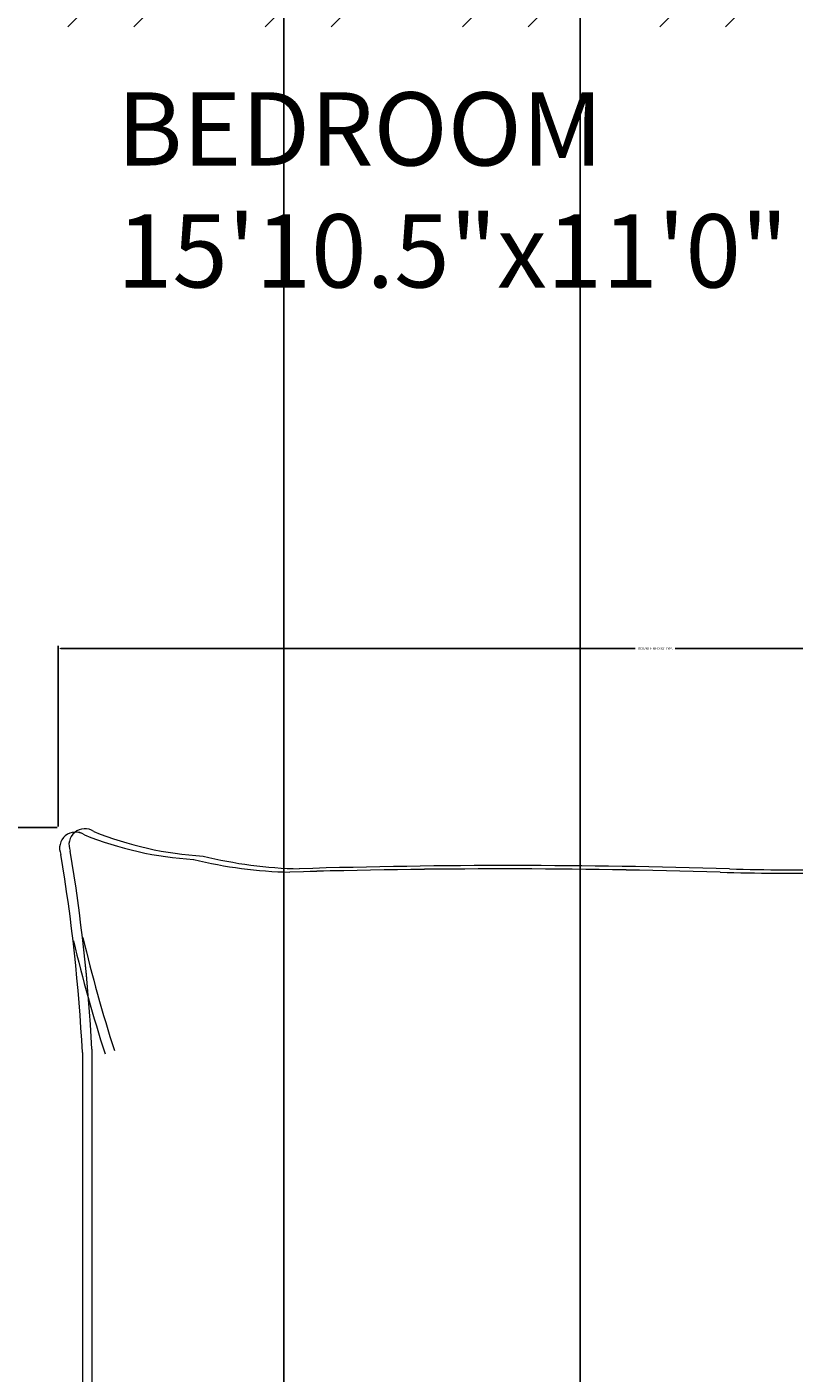
# Model space of a CAD drawing. Units: inches. Extents: x 1601 to 2297, y 1496 to 2631.
# Tile 21 of 57: x 2140 to 2193, y 1701 to 1793. Entities that reach past the tile are written whole.
import ezdxf

# ---------------------------------------------------------------- set-up
doc = ezdxf.new("R2010")
doc.units = ezdxf.units.IN
for name, color, linetype, lineweight in [('A-ANNO-DIMS', 2, 'Continuous', 18), ('A-AREA-IDEN', 7, 'Continuous', 18), ('A-FURN', 8, 'Continuous', 18), ('A-WALL-PATT', 215, 'Continuous', 13)]:
    doc.layers.add(name, color=color, linetype=linetype, lineweight=lineweight)
doc.styles.get("Standard").update_dxf_attribs({"font": 'arial.ttf'})
doc.dimstyles.get("Standard").update_dxf_attribs({"dimtxt": 0.18, "dimasz": 0.18, "dimexe": 0.18, "dimexo": 0.0625, "dimgap": 0.09, "dimtad": 0, "dimtih": 1, "dimtoh": 1, "dimdec": 4, "dimzin": 0, "dimdsep": 46, "dimtxsty": 'Standard', "dimcen": 0.09, "dimadec": 0, "dimazin": 0, "dimtfac": 1, "dimtdec": 4, "dimtofl": 0, "dimtmove": 0, "dimatfit": 3, "dimfxl": 1, "dimtolj": 1, "dimtzin": 0, "dimarcsym": 0})

# ---------------------------------------------------------------- blocks, each defined once
blk = doc.blocks.new('BED-DOUBLE')
for p, q in [((79.245, 15.063), (79.245, 39.677)), ((79.245, 15.063), (79.245, 39.677)), ((79.245, 15.063), (79.245, 39.677)), ((79.245, 15.063), (79.245, 39.677)), ((79.884, 15.292), (79.884, 39.905)), ((79.884, 15.291), (79.884, 39.905)), ((79.884, 15.292), (79.884, 39.905)), ((79.884, 15.291), (79.884, 39.905))]:
    blk.add_line(p, q)
for centre, radius, start, end in [((-23.712, -17.222), 106.459, 13.38322, 17.70533), ((-23.712, -17.222), 106.459, 13.38322, 17.70533), ((-23.712, -17.222), 106.459, 13.38322, 17.70533), ((-23.712, -17.222), 106.459, 13.38322, 17.70533), ((-23.073, -16.994), 106.459, 13.38322, 17.70533), ((-23.073, -16.994), 106.459, 13.38322, 17.70533), ((-23.073, -16.994), 106.459, 13.38322, 17.70533), ((-23.073, -16.994), 106.459, 13.38322, 17.70533), ((200.837, 21.427), 121.759, 182.99578, 189.40907), ((200.837, 21.426), 121.759, 182.99578, 189.40907), ((200.837, 21.427), 121.759, 182.99578, 189.40907), ((200.837, 21.426), 121.759, 182.99578, 189.40907), ((201.476, 21.655), 121.759, 182.99578, 189.40907), ((201.476, 21.655), 121.759, 182.99578, 189.40907), ((201.476, 21.655), 121.759, 182.99578, 189.40907), ((201.476, 21.655), 121.759, 182.99578, 189.40907), ((31.174, -167.308), 170.11, 88.4762, 91.00819), ((31.174, -167.308), 170.11, 88.4762, 91.00819), ((31.174, -167.308), 170.11, 88.4762, 91.00819), ((31.174, -167.308), 170.11, 88.4762, 91.00819), ((31.813, -167.079), 170.11, 88.4762, 91.00819), ((31.813, -167.08), 170.11, 88.4762, 91.00819), ((31.813, -167.079), 170.11, 88.4762, 91.00819), ((31.813, -167.08), 170.11, 88.4762, 91.00819), ((51.253, 485.051), 482.31, 268.22771, 271.71854), ((51.253, 485.05), 482.31, 268.22771, 271.71854), ((51.253, 485.051), 482.31, 268.22771, 271.71854), ((51.253, 485.05), 482.31, 268.22771, 271.71854), ((65.154, -26.671), 29.634, 76.06484, 88.91125), ((65.154, -26.672), 29.634, 76.06484, 88.91125), ((65.154, -26.671), 29.634, 76.06484, 88.91125), ((65.154, -26.672), 29.634, 76.06484, 88.91125), ((50.614, 484.822), 482.31, 268.22771, 271.71854), ((50.614, 484.822), 482.31, 268.22771, 271.71854), ((50.614, 484.822), 482.31, 268.22771, 271.71854), ((50.614, 484.822), 482.31, 268.22771, 271.71854), ((64.515, -26.9), 29.634, 76.06484, 88.91125), ((64.515, -26.9), 29.634, 76.06484, 88.91125), ((64.515, -26.9), 29.634, 76.06484, 88.91125), ((64.515, -26.9), 29.634, 76.06484, 88.91125), ((70.276, -21.66), 23.562, 67.97508, 86.652), ((70.276, -21.66), 23.562, 67.97508, 86.652), ((70.276, -21.66), 23.562, 67.97508, 86.652), ((70.276, -21.66), 23.562, 67.97508, 86.652), ((70.915, -21.431), 23.562, 67.97508, 86.652), ((70.915, -21.432), 23.562, 67.97508, 86.652), ((70.915, -21.431), 23.562, 67.97508, 86.652), ((70.915, -21.432), 23.562, 67.97508, 86.652), ((79.718, 1.087), 1.089, 236.17358, 23.47814), ((79.718, 1.087), 1.089, 236.17358, 23.47814), ((79.718, 1.087), 1.089, 236.17358, 23.47814), ((79.718, 1.087), 1.089, 236.17358, 23.47814), ((80.357, 1.316), 1.089, 236.17358, 23.47814), ((80.357, 1.316), 1.089, 236.17358, 23.47814), ((80.357, 1.315), 1.089, 236.17358, 23.47814), ((80.357, 1.315), 1.089, 236.17358, 23.47814)]:
    blk.add_arc(centre, radius, start, end)
blk = doc.blocks.new('*D12')
at = {"layer": 'A-ANNO-DIMS', "color": 0, "lineweight": -2, "transparency": 16777216}
for p, q in [((2142.379, 1738.191), (2142.379, 1750.54)), ((2142.559, 1750.36), (2181.784, 1750.36)), ((2223.747, 1750.36), (2184.522, 1750.36)), ((2223.927, 1738.191), (2223.927, 1750.54))]:
    blk.add_line(p, q, dxfattribs=at)
at = {"layer": 'A-ANNO-DIMS', "color": 0, "transparency": 16777216}
for points in [[(2142.559, 1750.39), (2142.559, 1750.33), (2142.379, 1750.36)], [(2223.747, 1750.39), (2223.747, 1750.33), (2223.927, 1750.36)]]:
    blk.add_solid(points, dxfattribs=at)
at = {"layer": 'Defpoints', "color": 0, "transparency": 16777216}
for p in [(2142.379, 1750.36), (2142.379, 1738.128), (2223.927, 1738.128)]:
    blk.add_point(p, dxfattribs=at)
at = {"layer": 'A-ANNO-DIMS', "color": 0, "transparency": 16777216, "insert": (2183.153, 1750.36), "char_height": 0.18, "attachment_point": 5}
blk.add_mtext('\\A1;DOUBLE BED 82 TYP.', dxfattribs=at)
blk = doc.blocks.new('*D13')
at = {"layer": 'A-ANNO-DIMS', "color": 0, "lineweight": -2, "transparency": 16777216}
for p, q in [((2142.316, 1738.128), (2129.966, 1738.128)), ((2130.146, 1737.948), (2130.146, 1710.398)), ((2130.146, 1682.484), (2130.146, 1710.034)), ((2142.316, 1682.304), (2129.966, 1682.304))]:
    blk.add_line(p, q, dxfattribs=at)
at = {"layer": 'A-ANNO-DIMS', "color": 0, "transparency": 16777216}
for points in [[(2130.116, 1737.948), (2130.176, 1737.948), (2130.146, 1738.128)], [(2130.116, 1682.484), (2130.176, 1682.484), (2130.146, 1682.304)]]:
    blk.add_solid(points, dxfattribs=at)
at = {"layer": 'Defpoints', "color": 0, "transparency": 16777216}
for p in [(2142.379, 1738.128), (2130.146, 1682.304), (2142.379, 1682.304)]:
    blk.add_point(p, dxfattribs=at)
at = {"layer": 'A-ANNO-DIMS', "color": 0, "transparency": 16777216, "insert": (2130.146, 1710.216), "char_height": 0.18, "attachment_point": 5}
blk.add_mtext('\\A1;56 TYP.', dxfattribs=at)
blk = doc.blocks.new('*D38')
at = {"layer": 'A-ANNO-DIMS', "color": 0, "lineweight": -2, "transparency": 16777216}
for p, q in [((2178.037, 2085.263), (2178.037, 1513.748)), ((2157.799, 2066.513), (2157.799, 1513.748)), ((2157.979, 1513.928), (2167.523, 1513.928)), ((2177.857, 1513.928), (2168.313, 1513.928))]:
    blk.add_line(p, q, dxfattribs=at)
at = {"layer": 'A-ANNO-DIMS', "color": 0, "transparency": 16777216}
for points in [[(2157.979, 1513.958), (2157.979, 1513.898), (2157.799, 1513.928)], [(2177.857, 1513.958), (2177.857, 1513.898), (2178.037, 1513.928)]]:
    blk.add_solid(points, dxfattribs=at)
at = {"layer": 'Defpoints', "color": 0, "transparency": 16777216}
for p in [(2178.037, 2085.325), (2157.799, 2066.575), (2178.037, 1513.928)]:
    blk.add_point(p, dxfattribs=at)
at = {"layer": 'A-ANNO-DIMS', "color": 0, "transparency": 16777216, "insert": (2167.918, 1513.928), "char_height": 0.18, "attachment_point": 5}
blk.add_mtext('\\A1;20.24', dxfattribs=at)

msp = doc.modelspace()

# ---------------------------------------------------------------- hatches: boundary and pattern name
at = {"layer": 'A-WALL-PATT'}
h = msp.add_hatch(dxfattribs=at)
h.set_pattern_fill('ANSI32', color=256)
h.paths.add_polyline_path([(1842.0336, 2528.0767), (1842.0336, 2532.3254), (1686.0373, 2532.3254), (1686.0373, 2492.9493), (1695.0373, 2492.9493), (1695.0373, 2523.3254), (1827.0373, 2523.3254), (1827.0373, 2416.8254), (1834.6225, 2416.8254), (1834.6225, 2419.0754), (1834.6225, 2421.3254), (1831.5373, 2421.3254), (1831.5373, 2523.3254), (1842.0336, 2523.3254)])
h.paths.add_polyline_path([(1695.0373, 2432.9493), (1686.0373, 2432.9493), (1686.0373, 2325.989), (1695.0373, 2325.989), (1695.0373, 2347.8254), (1827.0373, 2347.8254), (1827.0373, 2287.8254), (1823.2991, 2287.8254), (1823.2991, 2283.3254), (1847.9422, 2283.3254), (1847.9422, 2285.5754), (1847.9422, 2287.8254), (1831.5373, 2287.8254), (1831.5373, 2347.8254), (1846.9946, 2347.8254), (1846.9946, 2350.0754), (1846.9946, 2352.3254), (1695.0373, 2352.3254)])
h.paths.add_polyline_path([(1807.1169, 1573.5395), (2055.0405, 1573.5395), (2055.0405, 1610.6322), (1807.1169, 1610.6322)], flags=9)
h.paths.add_polyline_path([(1841.1631, 1712.7967), (1870.3957, 1712.7967), (1870.3957, 1731.454), (1841.1631, 1731.454)], flags=9)
h.paths.add_polyline_path([(2144.3862, 1772.185), (2191.0233, 1772.185), (2191.0233, 1790.8423), (2144.3862, 1790.8423)], flags=9)
h.paths.add_polyline_path([(2143.0128, 1827.3312), (2177.9958, 1827.3312), (2177.9958, 1845.9886), (2143.0128, 1845.9886)], flags=9)
h.paths.add_polyline_path([(2041.2439, 1833.5691), (2070.8516, 1833.5691), (2070.8516, 1852.2264), (2041.2439, 1852.2264)], flags=9)
h.paths.add_polyline_path([(2097.2791, 1947.0598), (2134.2061, 1947.0598), (2134.2061, 1965.7171), (2097.2791, 1965.7171)], flags=9)
h.paths.add_polyline_path([(2214.995, 1904.3124), (2214.995, 1942.2899), (2196.3376, 1942.2899), (2196.3376, 1904.3124)], flags=9)
h.paths.add_polyline_path([(2186.6284, 2043.8031), (2219.7935, 2043.8031), (2219.7935, 2062.4605), (2186.6284, 2062.4605)], flags=9)
h.paths.add_polyline_path([(2064.0877, 2031.616), (2097.4949, 2031.616), (2097.4949, 2050.2734), (2064.0877, 2050.2734)], flags=9)
h.paths.add_polyline_path([(1973.1349, 1986.0688), (2008.4009, 1986.0688), (2008.4009, 2004.7261), (1973.1349, 2004.7261)], flags=9)
h.paths.add_polyline_path([(1976.3676, 2106.9635), (2005.7469, 2106.9635), (2005.7469, 2125.6209), (1976.3676, 2125.6209)], flags=9)
h.paths.add_polyline_path([(1991.7852, 2180.4863), (2027.0513, 2180.4863), (2027.0513, 2199.1437), (1991.7852, 2199.1437)], flags=9)
h.paths.add_polyline_path([(2106.1801, 2187.9359), (2152.2101, 2187.9359), (2152.2101, 2206.5932), (2106.1801, 2206.5932)], flags=9)
h.paths.add_polyline_path([(2148.6686, 2262.2542), (2182.318, 2262.2542), (2182.318, 2280.9115), (2148.6686, 2280.9115)], flags=9)
h.paths.add_polyline_path([(2041.6327, 2252.8147), (2071.2405, 2252.8147), (2071.2405, 2271.4721), (2041.6327, 2271.4721)], flags=9)
h.paths.add_polyline_path([(2063.9734, 2375.4265), (2100.9004, 2375.4265), (2100.9004, 2394.0839), (2063.9734, 2394.0839)], flags=9)
h.paths.add_polyline_path([(2216.4955, 2330.9748), (2216.4955, 2370.2654), (2197.8381, 2370.2654), (2197.8381, 2330.9748)], flags=9)
h.paths.add_polyline_path([(2179.1416, 2485.8687), (2212.3067, 2485.8687), (2212.3067, 2504.5261), (2179.1416, 2504.5261)], flags=9)
h.paths.add_polyline_path([(2078.7442, 2471.1516), (2112.1514, 2471.1516), (2112.1514, 2489.809), (2078.7442, 2489.809)], flags=9)
h.paths.add_polyline_path([(1915.9631, 2329.4668), (1952.8902, 2329.4668), (1952.8902, 2348.1241), (1915.9631, 2348.1241)], flags=9)
h.paths.add_polyline_path([(1904.3189, 2499.6709), (1940.4512, 2499.6709), (1940.4512, 2518.3282), (1904.3189, 2518.3282)], flags=9)
h.paths.add_polyline_path([(1892.3665, 2100.4595), (1925.6374, 2100.4595), (1925.6374, 2119.1169), (1892.3665, 2119.1169)], flags=9)
h.paths.add_polyline_path([(1909.2984, 1805.9631), (1946.2254, 1805.9631), (1946.2254, 1824.6205), (1909.2984, 1824.6205)], flags=9)
h.paths.add_polyline_path([(1934.6056, 1658.616), (1970.738, 1658.616), (1970.738, 1677.2733), (1934.6056, 1677.2733)], flags=9)
h.paths.add_polyline_path([(1711.2052, 1789.8902), (1750.0456, 1789.8902), (1750.0456, 1808.5476), (1711.2052, 1808.5476)], flags=9)
h.paths.add_polyline_path([(1742.7874, 1854.6743), (1771.9449, 1854.6743), (1771.9449, 1873.3317), (1742.7874, 1873.3317)], flags=9)
h.paths.add_polyline_path([(1807.3592, 1997.7912), (1850.1116, 1997.7912), (1850.1116, 2016.4486), (1807.3592, 2016.4486)], flags=9)
h.paths.add_polyline_path([(1717.4579, 2237.7844), (1760.2103, 2237.7844), (1760.2103, 2256.4417), (1717.4579, 2256.4417)], flags=9)
h.paths.add_polyline_path([(1780.9285, 2324.0623), (1810.086, 2324.0623), (1810.086, 2342.7197), (1780.9285, 2342.7197)], flags=25)
h.paths.add_polyline_path([(1837.696, 2449.2024), (1866.9286, 2449.2024), (1866.9286, 2467.8598), (1837.696, 2467.8598)], flags=9)
h.paths.add_polyline_path([(1712.7752, 2484.9404), (1751.6156, 2484.9404), (1751.6156, 2503.5977), (1712.7752, 2503.5977)], flags=25)
h = msp.add_hatch(dxfattribs=at)
h.set_pattern_fill('ANSI32', color=256)
h.paths.add_polyline_path([(1973.9371, 2211.3254), (1893.0373, 2211.3254), (1893.0373, 2287.8254), (1884.6167, 2287.8254), (1884.6167, 2285.5754), (1884.6167, 2283.3254), (1888.5373, 2283.3254), (1888.5373, 2145.3254), (1695.0373, 2145.3254), (1695.0373, 2173.8724), (1690.5373, 2173.8724), (1686.0373, 2173.8724), (1686.0373, 2136.3254), (1722.5687, 2136.3254), (1722.5687, 2117.4352), (1731.5687, 2117.4352), (1731.5687, 2136.3254), (1893.0373, 2136.3254), (1893.0373, 2202.3254), (1959.0373, 2202.3254), (1959.0373, 2182.1303), (1968.0373, 2182.1303), (1968.0373, 2202.3254), (1973.9371, 2202.3254)])
h.paths.add_polyline_path([(2094.0373, 2274.6364), (2096.4294, 2274.6364), (2096.4294, 2276.8864), (2096.4294, 2279.1364), (2094.0373, 2279.1364), (2094.0373, 2290.8254), (2094.0373, 2295.3254), (2089.5373, 2295.3254), (2089.5373, 2230.8254), (2035.5373, 2230.8254), (2035.5373, 2299.8254), (2031.0373, 2299.8254), (2031.0373, 2211.3254), (2023.0065, 2211.3254), (2023.0065, 2202.3254), (2031.0373, 2202.3254), (2031.0373, 2140.8254), (1968.0373, 2140.8254), (1968.0373, 2145.9106), (1963.5373, 2145.9106), (1959.0373, 2145.9106), (1959.0373, 2116.839), (1963.5373, 2116.839), (1968.0373, 2116.839), (1968.0373, 2131.8254), (2031.0373, 2131.8254), (2031.0373, 2094.3254), (2031.0373, 2085.3254), (2031.0373, 2056.8254), (1968.0373, 2056.8254), (1968.0373, 2070.4947), (1963.5373, 2070.4947), (1959.0373, 2070.4947), (1959.0373, 2040.3029), (1968.0373, 2040.3029), (1968.0373, 2047.8254), (2031.0373, 2047.8254), (2031.0373, 1983.3254), (2031.0373, 1978.8254), (2021.1979, 1978.8254), (2021.1979, 1974.3254), (2031.0373, 1974.3254), (2031.0373, 1954.3528), (2035.5373, 1954.3528), (2035.5373, 1974.3254), (2035.5373, 1981.8254), (2055.5513, 1981.8254), (2055.5513, 1986.3254), (2035.5373, 1986.3254), (2035.5373, 2047.8254), (2040.0373, 2047.8254), (2040.0373, 2085.3254), (2040.0373, 2094.3254), (2040.0373, 2140.8254), (2035.5373, 2140.8254), (2035.5373, 2226.3254), (2089.5373, 2226.3254), (2094.0373, 2226.3254)])
h.paths.add_polyline_path([(2226.0373, 2230.8254), (2134.5373, 2230.8254), (2134.5373, 2233.5437), (2130.0373, 2233.5437), (2130.0373, 2226.3254), (2134.5373, 2226.3254), (2226.0373, 2226.3254)])
h.paths.add_polyline_path([(1807.1169, 1573.5395), (2055.0405, 1573.5395), (2055.0405, 1610.6322), (1807.1169, 1610.6322)], flags=9)
h.paths.add_polyline_path([(1841.1631, 1712.7967), (1870.3957, 1712.7967), (1870.3957, 1731.454), (1841.1631, 1731.454)], flags=9)
h.paths.add_polyline_path([(2144.3862, 1772.185), (2191.0233, 1772.185), (2191.0233, 1790.8423), (2144.3862, 1790.8423)], flags=9)
h.paths.add_polyline_path([(2143.0128, 1827.3312), (2177.9958, 1827.3312), (2177.9958, 1845.9886), (2143.0128, 1845.9886)], flags=9)
h.paths.add_polyline_path([(2041.2439, 1833.5691), (2070.8516, 1833.5691), (2070.8516, 1852.2264), (2041.2439, 1852.2264)], flags=9)
h.paths.add_polyline_path([(2097.2791, 1947.0598), (2134.2061, 1947.0598), (2134.2061, 1965.7171), (2097.2791, 1965.7171)], flags=9)
h.paths.add_polyline_path([(2214.995, 1904.3124), (2214.995, 1942.2899), (2196.3376, 1942.2899), (2196.3376, 1904.3124)], flags=9)
h.paths.add_polyline_path([(2186.6284, 2043.8031), (2219.7935, 2043.8031), (2219.7935, 2062.4605), (2186.6284, 2062.4605)], flags=9)
h.paths.add_polyline_path([(2064.0877, 2031.616), (2097.4949, 2031.616), (2097.4949, 2050.2734), (2064.0877, 2050.2734)], flags=9)
h.paths.add_polyline_path([(1973.1349, 1986.0688), (2008.4009, 1986.0688), (2008.4009, 2004.7261), (1973.1349, 2004.7261)], flags=25)
h.paths.add_polyline_path([(1976.3676, 2106.9635), (2005.7469, 2106.9635), (2005.7469, 2125.6209), (1976.3676, 2125.6209)], flags=25)
h.paths.add_polyline_path([(1991.7852, 2180.4863), (2027.0513, 2180.4863), (2027.0513, 2199.1437), (1991.7852, 2199.1437)], flags=25)
h.paths.add_polyline_path([(2106.1801, 2187.9359), (2152.2101, 2187.9359), (2152.2101, 2206.5932), (2106.1801, 2206.5932)], flags=9)
h.paths.add_polyline_path([(2148.6686, 2262.2542), (2182.318, 2262.2542), (2182.318, 2280.9115), (2148.6686, 2280.9115)], flags=9)
h.paths.add_polyline_path([(2041.6327, 2252.8147), (2071.2405, 2252.8147), (2071.2405, 2271.4721), (2041.6327, 2271.4721)], flags=25)
h.paths.add_polyline_path([(2063.9734, 2375.4265), (2100.9004, 2375.4265), (2100.9004, 2394.0839), (2063.9734, 2394.0839)], flags=9)
h.paths.add_polyline_path([(2216.4955, 2330.9748), (2216.4955, 2370.2654), (2197.8381, 2370.2654), (2197.8381, 2330.9748)], flags=9)
h.paths.add_polyline_path([(2179.1416, 2485.8687), (2212.3067, 2485.8687), (2212.3067, 2504.5261), (2179.1416, 2504.5261)], flags=9)
h.paths.add_polyline_path([(2078.7442, 2471.1516), (2112.1514, 2471.1516), (2112.1514, 2489.809), (2078.7442, 2489.809)], flags=9)
h.paths.add_polyline_path([(1915.9631, 2329.4668), (1952.8902, 2329.4668), (1952.8902, 2348.1241), (1915.9631, 2348.1241)], flags=9)
h.paths.add_polyline_path([(1904.3189, 2499.6709), (1940.4512, 2499.6709), (1940.4512, 2518.3282), (1904.3189, 2518.3282)], flags=9)
h.paths.add_polyline_path([(1892.3665, 2100.4595), (1925.6374, 2100.4595), (1925.6374, 2119.1169), (1892.3665, 2119.1169)], flags=9)
h.paths.add_polyline_path([(1909.2984, 1805.9631), (1946.2254, 1805.9631), (1946.2254, 1824.6205), (1909.2984, 1824.6205)], flags=9)
h.paths.add_polyline_path([(1934.6056, 1658.616), (1970.738, 1658.616), (1970.738, 1677.2733), (1934.6056, 1677.2733)], flags=9)
h.paths.add_polyline_path([(1711.2052, 1789.8902), (1750.0456, 1789.8902), (1750.0456, 1808.5476), (1711.2052, 1808.5476)], flags=9)
h.paths.add_polyline_path([(1742.7874, 1854.6743), (1771.9449, 1854.6743), (1771.9449, 1873.3317), (1742.7874, 1873.3317)], flags=9)
h.paths.add_polyline_path([(1807.3592, 1997.7912), (1850.1116, 1997.7912), (1850.1116, 2016.4486), (1807.3592, 2016.4486)], flags=9)
h.paths.add_polyline_path([(1717.4579, 2237.7844), (1760.2103, 2237.7844), (1760.2103, 2256.4417), (1717.4579, 2256.4417)], flags=25)
h.paths.add_polyline_path([(1780.9285, 2324.0623), (1810.086, 2324.0623), (1810.086, 2342.7197), (1780.9285, 2342.7197)], flags=9)
h.paths.add_polyline_path([(1837.696, 2449.2024), (1866.9286, 2449.2024), (1866.9286, 2467.8598), (1837.696, 2467.8598)], flags=9)
h.paths.add_polyline_path([(1712.7752, 2484.9404), (1751.6156, 2484.9404), (1751.6156, 2503.5977), (1712.7752, 2503.5977)], flags=9)
h = msp.add_hatch(dxfattribs=at)
h.set_pattern_fill('ANSI32', color=256)
h.paths.add_polyline_path([(2230.5373, 1861.8254), (2182.5373, 1861.8254), (2182.5373, 1885.3637), (2178.0373, 1885.3637), (2178.0373, 1861.8254), (2166.0373, 1861.8254), (2134.5373, 1861.8254), (2130.0373, 1861.8254), (2130.0373, 1841.4682), (2126.8833, 1841.4682), (2126.8833, 1836.9682), (2130.0373, 1836.9682), (2130.0373, 1822.7302), (2134.5373, 1822.7302), (2134.5373, 1857.3254), (2166.0373, 1857.3254), (2226.0373, 1857.3254), (2226.0373, 1846.1155), (2230.5373, 1846.1155)])
h.paths.add_polyline_path([(2226.0373, 1797.3254), (2134.5373, 1797.3254), (2134.5373, 1800.6636), (2132.2873, 1800.6636), (2130.0373, 1800.6636), (2130.0373, 1797.3254), (2130.0373, 1792.8254), (2167.7264, 1792.8254), (2226.0373, 1792.8254)])
h.paths.add_polyline_path([(2230.5373, 1822.1155), (2226.0373, 1822.1155), (2226.0373, 1760.8563), (2230.5373, 1760.8563)])
h.paths.add_polyline_path([(2230.5373, 1700.8563), (2226.0373, 1700.8563), (2226.0373, 1644.3254), (2140.2517, 1644.3254), (2140.2517, 1635.3254), (2230.5373, 1635.3254)])
h.paths.add_polyline_path([(2080.2517, 1639.8254), (2080.2517, 1644.3254), (2035.5373, 1644.3254), (2035.5373, 1792.8254), (2094.0373, 1792.8254), (2094.0373, 1797.3254), (2094.0373, 1836.9682), (2097.1057, 1836.9682), (2097.1057, 1839.2182), (2097.1057, 1841.4682), (2094.0373, 1841.4682), (2094.0373, 1862.2276), (2089.5373, 1862.2276), (2089.5373, 1797.3254), (2035.5373, 1797.3254), (2035.5373, 1857.3254), (2035.5373, 1885.0916), (2031.0373, 1885.0916), (2031.0373, 1710.3254), (2012.329, 1710.3254), (2012.329, 1701.3254), (2031.0373, 1701.3254), (2031.0373, 1644.3254), (2031.0373, 1635.3254), (2080.2517, 1635.3254)])
h.paths.add_polyline_path([(1836.0373, 1653.2033), (1842.6171, 1653.2033), (1842.6171, 1657.7033), (1842.6171, 1662.2033), (1831.5373, 1662.2033), (1831.5373, 1764.2033), (1835.3881, 1764.2033), (1835.3881, 1766.4533), (1835.3881, 1768.7033), (1831.5373, 1768.7033), (1827.0373, 1768.7033), (1827.0373, 1662.2033), (1827.0373, 1635.3254), (1836.0373, 1635.3254)])
h.paths.add_polyline_path([(1893.0373, 1701.3254), (1907.193, 1701.3254), (1907.193, 1705.8254), (1907.193, 1710.3254), (1893.0373, 1710.3254), (1893.0373, 1819.8254), (1882.6444, 1819.8254), (1882.6444, 1817.5754), (1882.6444, 1815.3254), (1888.5373, 1815.3254), (1888.5373, 1662.2033), (1884.0373, 1662.2033), (1866.6171, 1662.2033), (1866.6171, 1653.2033), (1882.391, 1653.2033), (1884.0373, 1653.2033), (1884.0373, 1635.3254), (1893.0373, 1635.3254)])
h.paths.add_polyline_path([(1739.3335, 1639.8254), (1739.3335, 1644.3254), (1695.0373, 1644.3254), (1695.0373, 1702.0135), (1690.5373, 1702.0135), (1686.0373, 1702.0135), (1686.0373, 1635.3254), (1739.3335, 1635.3254)])
h.paths.add_polyline_path([(1827.0373, 1644.3254), (1799.3335, 1644.3254), (1799.3335, 1635.3254), (1827.0373, 1635.3254)])
h.paths.add_polyline_path([(1695.0373, 1815.3254), (1849.2759, 1815.3254), (1849.2759, 1819.8254), (1807.5373, 1819.8254), (1807.5373, 1879.8254), (1851.1533, 1879.8254), (1851.1533, 1882.0754), (1851.1533, 1884.3254), (1799.3405, 1884.3254), (1799.3405, 1882.0754), (1799.3405, 1879.8254), (1803.0373, 1879.8254), (1803.0373, 1819.8254), (1695.0373, 1819.8254), (1695.0373, 1835.0458), (1690.5373, 1835.0458), (1686.0373, 1835.0458), (1686.0373, 1766.1753), (1695.0373, 1766.1753)])
h.paths.add_polyline_path([(1775.8157, 1884.3254), (1695.0373, 1884.3254), (1695.0373, 1912.9526), (1690.5373, 1912.9526), (1686.0373, 1912.9526), (1686.0373, 1859.0458), (1695.0373, 1859.0458), (1695.0373, 1879.8254), (1775.8157, 1879.8254)])
h.paths.add_polyline_path([(1893.0373, 2031.3254), (1731.5687, 2031.3254), (1731.5687, 2057.4352), (1722.5687, 2057.4352), (1722.5687, 2031.3254), (1686.0373, 2031.3254), (1686.0373, 1972.9526), (1695.0373, 1972.9526), (1695.0373, 2022.3254), (1888.5373, 2022.3254), (1888.5373, 1884.3254), (1883.4996, 1884.3254), (1883.4996, 1879.8254), (1893.0373, 1879.8254), (1893.0373, 1974.3254), (1976.6199, 1974.3254), (1976.6199, 1978.8254), (1968.0373, 1978.8254), (1968.0373, 1983.3254), (1968.0373, 2008.4756), (1963.5373, 2008.4756), (1959.0373, 2008.4756), (1959.0373, 1983.3254), (1893.0373, 1983.3254)])
h.paths.add_polyline_path([(2230.5373, 2140.4745), (2226.0373, 2140.4745), (2226.0373, 2094.3254), (2040.0373, 2094.3254), (2040.0373, 2085.3254), (2178.0373, 2085.3254), (2178.0373, 2065.6965), (2182.5373, 2065.6965), (2182.5373, 2085.3254), (2226.0373, 2085.3254), (2226.0373, 1986.3254), (2211.2679, 1986.3254), (2211.2679, 1981.8254), (2230.5373, 1981.8254)])
h.paths.add_polyline_path([(2187.6292, 1986.3254), (2182.5373, 1986.3254), (2182.5373, 2029.6965), (2178.0373, 2029.6965), (2178.0373, 1986.3254), (2099.05, 1986.3254), (2099.05, 1981.8254), (2178.0373, 1981.8254), (2178.0373, 1969.3637), (2182.5373, 1969.3637), (2182.5373, 1981.8254), (2187.6292, 1981.8254), (2187.6292, 1984.0754)])
h.paths.add_polyline_path([(1807.1169, 1573.5395), (2055.0405, 1573.5395), (2055.0405, 1610.6322), (1807.1169, 1610.6322)], flags=9)
h.paths.add_polyline_path([(1841.1631, 1712.7967), (1870.3957, 1712.7967), (1870.3957, 1731.454), (1841.1631, 1731.454)], flags=9)
h.paths.add_polyline_path([(2144.3862, 1772.185), (2191.0233, 1772.185), (2191.0233, 1790.8423), (2144.3862, 1790.8423)], flags=9)
h.paths.add_polyline_path([(2143.0128, 1827.3312), (2177.9958, 1827.3312), (2177.9958, 1845.9886), (2143.0128, 1845.9886)], flags=25)
h.paths.add_polyline_path([(2041.2439, 1833.5691), (2070.8516, 1833.5691), (2070.8516, 1852.2264), (2041.2439, 1852.2264)], flags=25)
h.paths.add_polyline_path([(2097.2791, 1947.0598), (2134.2061, 1947.0598), (2134.2061, 1965.7171), (2097.2791, 1965.7171)], flags=9)
h.paths.add_polyline_path([(2214.995, 1904.3124), (2214.995, 1942.2899), (2196.3376, 1942.2899), (2196.3376, 1904.3124)], flags=9)
h.paths.add_polyline_path([(2186.6284, 2043.8031), (2219.7935, 2043.8031), (2219.7935, 2062.4605), (2186.6284, 2062.4605)], flags=25)
h.paths.add_polyline_path([(2064.0877, 2031.616), (2097.4949, 2031.616), (2097.4949, 2050.2734), (2064.0877, 2050.2734)], flags=25)
h.paths.add_polyline_path([(1973.1349, 1986.0688), (2008.4009, 1986.0688), (2008.4009, 2004.7261), (1973.1349, 2004.7261)], flags=9)
h.paths.add_polyline_path([(1976.3676, 2106.9635), (2005.7469, 2106.9635), (2005.7469, 2125.6209), (1976.3676, 2125.6209)], flags=9)
h.paths.add_polyline_path([(1991.7852, 2180.4863), (2027.0513, 2180.4863), (2027.0513, 2199.1437), (1991.7852, 2199.1437)], flags=9)
h.paths.add_polyline_path([(2106.1801, 2187.9359), (2152.2101, 2187.9359), (2152.2101, 2206.5932), (2106.1801, 2206.5932)], flags=9)
h.paths.add_polyline_path([(2148.6686, 2262.2542), (2182.318, 2262.2542), (2182.318, 2280.9115), (2148.6686, 2280.9115)], flags=9)
h.paths.add_polyline_path([(2041.6327, 2252.8147), (2071.2405, 2252.8147), (2071.2405, 2271.4721), (2041.6327, 2271.4721)], flags=9)
h.paths.add_polyline_path([(2063.9734, 2375.4265), (2100.9004, 2375.4265), (2100.9004, 2394.0839), (2063.9734, 2394.0839)], flags=9)
h.paths.add_polyline_path([(2216.4955, 2330.9748), (2216.4955, 2370.2654), (2197.8381, 2370.2654), (2197.8381, 2330.9748)], flags=9)
h.paths.add_polyline_path([(2179.1416, 2485.8687), (2212.3067, 2485.8687), (2212.3067, 2504.5261), (2179.1416, 2504.5261)], flags=9)
h.paths.add_polyline_path([(2078.7442, 2471.1516), (2112.1514, 2471.1516), (2112.1514, 2489.809), (2078.7442, 2489.809)], flags=9)
h.paths.add_polyline_path([(1915.9631, 2329.4668), (1952.8902, 2329.4668), (1952.8902, 2348.1241), (1915.9631, 2348.1241)], flags=9)
h.paths.add_polyline_path([(1904.3189, 2499.6709), (1940.4512, 2499.6709), (1940.4512, 2518.3282), (1904.3189, 2518.3282)], flags=9)
h.paths.add_polyline_path([(1892.3665, 2100.4595), (1925.6374, 2100.4595), (1925.6374, 2119.1169), (1892.3665, 2119.1169)], flags=9)
h.paths.add_polyline_path([(1909.2984, 1805.9631), (1946.2254, 1805.9631), (1946.2254, 1824.6205), (1909.2984, 1824.6205)], flags=9)
h.paths.add_polyline_path([(1934.6056, 1658.616), (1970.738, 1658.616), (1970.738, 1677.2733), (1934.6056, 1677.2733)], flags=9)
h.paths.add_polyline_path([(1711.2052, 1789.8902), (1750.0456, 1789.8902), (1750.0456, 1808.5476), (1711.2052, 1808.5476)], flags=25)
h.paths.add_polyline_path([(1742.7874, 1854.6743), (1771.9449, 1854.6743), (1771.9449, 1873.3317), (1742.7874, 1873.3317)], flags=25)
h.paths.add_polyline_path([(1807.3592, 1997.7912), (1850.1116, 1997.7912), (1850.1116, 2016.4486), (1807.3592, 2016.4486)], flags=25)
h.paths.add_polyline_path([(1717.4579, 2237.7844), (1760.2103, 2237.7844), (1760.2103, 2256.4417), (1717.4579, 2256.4417)], flags=9)
h.paths.add_polyline_path([(1780.9285, 2324.0623), (1810.086, 2324.0623), (1810.086, 2342.7197), (1780.9285, 2342.7197)], flags=9)
h.paths.add_polyline_path([(1837.696, 2449.2024), (1866.9286, 2449.2024), (1866.9286, 2467.8598), (1837.696, 2467.8598)], flags=9)
h.paths.add_polyline_path([(1712.7752, 2484.9404), (1751.6156, 2484.9404), (1751.6156, 2503.5977), (1712.7752, 2503.5977)], flags=9)

# ---------------------------------------------------------------- block references
at = {"layer": 'A-FURN', "rotation": 180}
msp.add_blockref('BED-DOUBLE', (2223.9271, 1738.0414), dxfattribs=at)

# ---------------------------------------------------------------- texts
at = {"layer": 'A-AREA-IDEN', "insert": (2146.3967, 1788.3577), "char_height": 5, "attachment_point": 1}
msp.add_mtext_dynamic_manual_height_columns('BEDROOM\\P15\'10.5"x11\'0"', width=127.396617, gutter_width=12.5, heights=[0], dxfattribs=at)

# ---------------------------------------------------------------- dimensions: what is measured, and where the dimension line sits
at = {"layer": 'A-ANNO-DIMS'}
dim = msp.add_linear_dim(base=(2178.0373, 1513.9279), p1=(2157.799, 2066.5754), p2=(2178.0373, 2085.3254), dimstyle='Standard', override={"dimdec": 2, "dimlfac": 1, "dimrnd": 0, "dimzin": 0, "dimdsep": 46, "dimlunit": 2}, dxfattribs=at)
dim.commit()
dim.dimension.update_dxf_attribs({"geometry": '*D38', "text_midpoint": (2167.9181, 1513.9279)})
for base, p1, p2, angle, text, picture, middle in [((2142.3787, 1750.3604), (2223.9273, 1738.1281), (2142.3787, 1738.1281), 180, 'DOUBLE BED <> TYP.', '*D12', (2183.153, 1750.3604)), ((2130.1464, 1682.3035), (2142.3787, 1738.1281), (2142.3787, 1682.3035), 270, '<> TYP.', '*D13', (2130.1464, 1710.2158))]:
    dim = msp.add_linear_dim(base=base, p1=p1, p2=p2, angle=angle, text=text, dimstyle='Standard', override={"dimdec": 0, "dimlfac": 1, "dimrnd": 0, "dimzin": 0, "dimdsep": 46, "dimlunit": 2}, dxfattribs=at)
    dim.commit()
    dim.dimension.update_dxf_attribs({"geometry": picture, "text_midpoint": middle})

doc.saveas('drawing.dxf')
